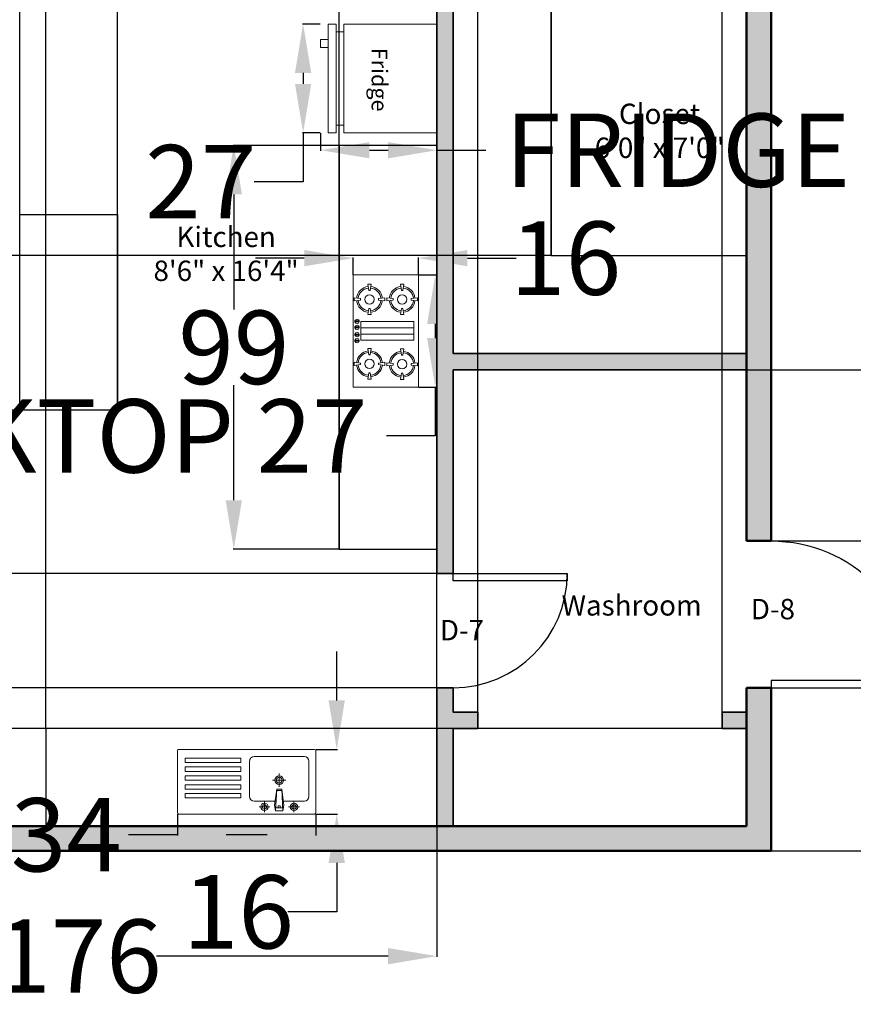
# Model space of a CAD drawing. Units: inches. Extents: x -478 to 256, y -93 to 343.
# Tile 3 of 5: x -106 to 98, y -93 to 149. Entities that reach past the tile are written whole.
import ezdxf

# ---------------------------------------------------------------- set-up
doc = ezdxf.new("R2010")
doc.units = ezdxf.units.IN
for name, color, linetype, lineweight in [('A-ANNO-DIMS', 2, 'Continuous', 18), ('A-ANNO-TEXT', 7, 'Continuous', 18), ('A-AREA-IDEN', 7, 'Continuous', 18), ('A-DOOR', 3, 'Continuous', 25), ('A-EQPM', 6, 'Continuous', 18), ('A-FLOR-CASE', 6, 'Continuous', 25), ('A-FLOR-FIXT', 9, 'Continuous', 18), ('A-WALL-PATT', 8, 'Continuous', 13), ('Inner Wall', 5, 'Continuous', 35), ('Outer Wall', 1, 'Continuous', 50)]:
    doc.layers.add(name, color=color, linetype=linetype, lineweight=lineweight)
doc.styles.get("Standard").update_dxf_attribs({"font": 'arial.ttf'})
doc.dimstyles.get("Standard").update_dxf_attribs({"dimtxt": 18, "dimasz": 12, "dimexe": 0.18, "dimexo": 0.0625, "dimgap": 0.09, "dimtad": 0, "dimtih": 1, "dimtoh": 1, "dimdec": 0, "dimzin": 0, "dimdsep": 46, "dimlunit": 3, "dimtxsty": 'Standard', "dimcen": 0.09, "dimadec": 0, "dimazin": 0, "dimtfac": 1, "dimtdec": 0, "dimtofl": 0, "dimtmove": 0, "dimatfit": 3, "dimfxl": 1, "dimtolj": 1, "dimtzin": 0, "dimarcsym": 0})

# ---------------------------------------------------------------- blocks, each defined once
blk = doc.blocks.new('REFRI-00')
for points in [[(-0.35, 0.35), (-0.35, -0.25), (0.35, -0.25), (0.35, 0.35), (-0.35, 0.35)], [(-0.3, -0.3), (-0.3, -0.25)], [(0.3, -0.3), (0.3, -0.25)], [(-0.35, -0.3), (-0.35, -0.35), (0.35, -0.35), (0.35, -0.3), (-0.35, -0.3)], [(-0.25, -0.35), (-0.25, -0.4), (-0.2, -0.4), (-0.2, -0.35)]]:
    blk.add_lwpolyline(points)
blk = doc.blocks.new('A$C57CF26DA')
for p, q in [((0, 0), (0, 420)), ((720, 420), (0, 420)), ((166.9, 413), (146.9, 413)), ((146.9, 413), (151.9, 373)), ((161.9, 373), (166.9, 413)), ((300, 390.9), (300, 49.1)), ((300, 390.9), (420, 390.9)), ((340, 390.9), (340, 49.1)), ((380, 390.9), (380, 49.1)), ((420, 390.9), (420, 49.1)), ((583.6, 413), (563.6, 413)), ((563.6, 413), (568.6, 373)), ((578.6, 373), (583.6, 413)), ((720, 0), (720, 420)), ((98.9, 320), (58.9, 325)), ((58.9, 325), (58.9, 305)), ((98.9, 310), (98.9, 320)), ((151.9, 373), (161.9, 373)), ((254.8, 325), (214.8, 320)), ((214.8, 320), (214.8, 310)), ((254.8, 305), (254.8, 325)), ((515.6, 320), (475.6, 325)), ((475.6, 325), (475.6, 305)), ((515.6, 310), (515.6, 320)), ((568.6, 373), (578.6, 373)), ((671.6, 325), (631.6, 320)), ((631.6, 320), (631.6, 310)), ((671.6, 305), (671.6, 325)), ((58.9, 305), (98.9, 310)), ((151.9, 257), (146.9, 217)), ((161.9, 257), (151.9, 257)), ((166.9, 217), (161.9, 257)), ((214.8, 310), (254.8, 305)), ((475.6, 305), (515.6, 310)), ((568.6, 257), (563.6, 217)), ((578.6, 257), (568.6, 257)), ((583.6, 217), (578.6, 257)), ((631.6, 310), (671.6, 305)), ((146.9, 217), (166.9, 217)), ((166.9, 203), (146.9, 203)), ((146.9, 203), (151.9, 163)), ((161.9, 163), (166.9, 203)), ((581.1, 203), (561.1, 203)), ((561.1, 203), (566.1, 163)), ((563.6, 217), (583.6, 217)), ((576.1, 163), (581.1, 203)), ((151.9, 163), (161.9, 163)), ((566.1, 163), (576.1, 163)), ((98.9, 110), (58.9, 115)), ((58.9, 115), (58.9, 95)), ((58.9, 95), (98.9, 100)), ((98.9, 100), (98.9, 110)), ((254.8, 115), (214.8, 110)), ((214.8, 110), (214.8, 100)), ((214.8, 100), (254.8, 95)), ((254.8, 95), (254.8, 115)), ((513.1, 110), (473.1, 115)), ((473.1, 115), (473.1, 95)), ((473.1, 95), (513.1, 100)), ((513.1, 100), (513.1, 110)), ((669, 115), (629, 110)), ((629, 110), (629, 100)), ((629, 100), (669, 95)), ((669, 95), (669, 115)), ((151.9, 47), (146.9, 7)), ((146.9, 7), (166.9, 7)), ((161.9, 47), (151.9, 47)), ((166.9, 7), (161.9, 47)), ((301.5, 38.7), (294.7, 38.7)), ((294.7, 38.7), (294.7, 11.3)), ((294.7, 11.3), (301.5, 11.3)), ((420, 49.1), (300, 49.1)), ((301.5, 11.3), (301.5, 38.7)), ((340.5, 38.7), (333.7, 38.7)), ((333.7, 38.7), (333.7, 11.3)), ((333.7, 11.3), (340.5, 11.3)), ((340.5, 11.3), (340.5, 38.7)), ((379.7, 11.3), (379.7, 38.7)), ((379.7, 38.7), (386.5, 38.7)), ((386.5, 11.3), (379.7, 11.3)), ((386.5, 38.7), (386.5, 11.3)), ((418.7, 11.3), (418.7, 38.7)), ((418.7, 38.7), (425.5, 38.7)), ((425.5, 11.3), (418.7, 11.3)), ((425.5, 38.7), (425.5, 11.3)), ((566.1, 47), (561.1, 7)), ((561.1, 7), (581.1, 7)), ((576.1, 47), (566.1, 47)), ((581.1, 7), (576.1, 47)), ((720, 0), (0, 0))]:
    blk.add_line(p, q)
for centre in [(156.9, 315), (573.6, 315), (156.9, 105), (571.1, 105)]:
    blk.add_circle(centre, 30)
for centre, radius, start, end in [((156.9, 315), 83, 95.58493, 174.41507), ((156.9, 315), 73, 95.37384, 174.62616), ((156.9, 315), 73, 5.37384, 84.62616), ((156.9, 315), 83, 5.58493, 84.41507), ((573.6, 315), 83, 95.58493, 174.41507), ((573.6, 315), 73, 95.37384, 174.62616), ((573.6, 315), 73, 5.37384, 84.62616), ((573.6, 315), 83, 5.58493, 84.41507), ((156.9, 315), 83, 185.58493, 264.41507), ((156.9, 315), 73, 185.37384, 264.62616), ((156.9, 315), 73, 275.37384, 354.62616), ((156.9, 315), 83, 275.58493, 354.41507), ((573.6, 315), 83, 185.58493, 264.41507), ((573.6, 315), 73, 185.37384, 264.62616), ((573.6, 315), 73, 275.37384, 354.62616), ((573.6, 315), 83, 275.58493, 354.41507), ((156.9, 105), 83, 95.58493, 174.41507), ((156.9, 105), 73, 95.37384, 174.62616), ((156.9, 105), 73, 5.37384, 84.62616), ((156.9, 105), 83, 5.58493, 84.41507), ((571.1, 105), 83, 95.58493, 174.41507), ((571.1, 105), 73, 95.37384, 174.62616), ((571.1, 105), 73, 5.37384, 84.62616), ((571.1, 105), 83, 5.58493, 84.41507), ((156.9, 105), 83, 185.58493, 264.41507), ((156.9, 105), 73, 185.37384, 264.62616), ((156.9, 105), 73, 275.37384, 354.62616), ((156.9, 105), 83, 275.58493, 354.41507), ((571.1, 105), 83, 185.58493, 264.41507), ((571.1, 105), 73, 185.37384, 264.62616), ((571.1, 105), 73, 275.37384, 354.62616), ((571.1, 105), 83, 275.58493, 354.41507), ((298.1, 25), 13.7, 104.47751, 255.52249), ((298.1, 25), 13.7, 284.47751, 75.52249), ((337.1, 25), 13.7, 104.47751, 255.52249), ((337.1, 25), 13.7, 284.47751, 75.52249), ((383.1, 25), 13.7, 104.47751, 255.52249), ((383.1, 25), 13.7, 284.47751, 75.52249), ((422.1, 25), 13.7, 104.47751, 255.52249), ((422.1, 25), 13.7, 284.47751, 75.52249)]:
    blk.add_arc(centre, radius, start, end)
blk = doc.blocks.new('A$C7C492201')
for p, q in [((0, 10), (0, 426.6)), ((10, 436.6), (927.3, 436.6)), ((148.5, 425.2), (148.5, 352.2)), ((223.5, 415), (217, 376.2)), ((223.5, 415), (231.8, 268.5)), ((223.5, 415), (248.5, 415)), ((273.5, 415), (248.5, 415)), ((273.5, 415), (265.2, 268.5)), ((273.5, 415), (279.9, 376.2)), ((348.5, 425.2), (348.5, 352.2)), ((937.3, 10), (937.3, 426.6)), ((220.8, 348.8), (78.5, 348.8)), ((111.9, 388.7), (185, 388.7)), ((217, 376.2), (231.8, 268.5)), ((224.6, 395.4), (248.5, 395.4)), ((272.3, 395.4), (248.5, 395.4)), ((279.9, 376.2), (265.2, 268.5)), ((418.5, 348.8), (276.2, 348.8)), ((311.9, 388.7), (385, 388.7)), ((48.5, 318.8), (48.5, 78.8)), ((231.3, 278.6), (248.5, 278.6)), ((231.8, 268.5), (248.5, 268.5)), ((265.6, 278.6), (248.5, 278.6)), ((265.2, 268.5), (248.5, 268.5)), ((448.5, 318.8), (448.5, 78.8)), ((509.1, 328.4), (509.1, 298.4)), ((509.1, 328.4), (885, 328.4)), ((509.1, 298.4), (885, 298.4)), ((509.1, 268.4), (509.1, 238.4)), ((509.1, 268.4), (885, 268.4)), ((885, 328.4), (885, 298.4)), ((885, 268.4), (885, 238.4)), ((203.4, 207.7), (293.5, 207.7)), ((248.5, 252.8), (248.5, 162.6)), ((509.1, 238.4), (885, 238.4)), ((509.1, 208.4), (885, 208.4)), ((509.1, 208.4), (509.1, 178.4)), ((885, 208.4), (885, 178.4)), ((509.1, 178.4), (885, 178.4)), ((509.1, 148.4), (509.1, 118.4)), ((509.1, 148.4), (885, 148.4)), ((885, 148.4), (885, 118.4)), ((509.1, 118.4), (885, 118.4)), ((509.1, 88.4), (509.1, 58.4)), ((509.1, 88.4), (885, 88.4)), ((885, 88.4), (885, 58.4)), ((927.3, 0), (10, 0)), ((418.5, 48.8), (78.5, 48.8)), ((509.1, 58.4), (885, 58.4))]:
    blk.add_line(p, q)
for centre, radius in [((148.5, 388.7), 25), ((148.5, 388.7), 15), ((348.5, 388.7), 25), ((348.5, 388.7), 15), ((248.5, 207.7), 30), ((248.5, 207.7), 20)]:
    blk.add_circle(centre, radius)
for centre, radius, start, end in [((10, 426.6), 10, 90, 180), ((927.3, 426.6), 10, 0, 90), ((78.5, 318.8), 30, 90, 180), ((247.3, 388), 7.19, 80.52523, 279.47477), ((249.6, 388), 7.19, 260.52523, 99.47477), ((418.5, 318.8), 30, 0, 90), ((78.5, 78.8), 30, 180, 270), ((418.5, 78.8), 30, 270, 0), ((10, 10), 10, 180, 270), ((927.3, 10), 10, 270, 0)]:
    blk.add_arc(centre, radius, start, end)
blk = doc.blocks.new('*U4')
for p, q in [((0, 0), (0, -4)), ((28, 0), (28, -4))]:
    blk.add_line(p, q)
blk.add_lwpolyline([(0, 0), (0, 28), (1.75, 28), (1.75, 0)], close=True)
blk.add_arc((0, 0), 28, 0, 90)
blk = doc.blocks.new('*U14')
for p, q in [((0, 0), (0, -6)), ((36, 0), (36, -6))]:
    blk.add_line(p, q)
blk.add_lwpolyline([(0, 0), (0, 36), (1.75, 36), (1.75, 0)], close=True)
blk.add_arc((0, 0), 36, 0, 90)
blk = doc.blocks.new('*D17')
at = {"layer": 'A-ANNO-DIMS', "color": 0, "lineweight": -2, "transparency": 16777216}
for p, q in [((-32.43, 120.92), (-32.43, 116.52)), ((-3.86, 120.92), (-3.86, 116.52)), ((-20.43, 116.7), (-15.86, 116.7)), ((-3.86, 116.7), (8.14, 116.7))]:
    blk.add_line(p, q, dxfattribs=at)
at = {"layer": 'A-ANNO-DIMS', "color": 0, "transparency": 16777216}
for points in [[(-20.43, 118.7), (-20.43, 114.7), (-32.43, 116.7)], [(-15.86, 118.7), (-15.86, 114.7), (-3.86, 116.7)]]:
    blk.add_solid(points, dxfattribs=at)
at = {"layer": 'Defpoints', "color": 0, "transparency": 16777216}
for p in [(-32.43, 120.98), (-3.86, 120.98), (-3.86, 116.7)]:
    blk.add_point(p, dxfattribs=at)
at = {"layer": 'A-ANNO-DIMS', "color": 0, "transparency": 16777216, "insert": (71.63, 116.7), "char_height": 18, "attachment_point": 5}
blk.add_mtext('\\A1;FRIDGE 29', dxfattribs=at)
blk = doc.blocks.new('*D18')
at = {"layer": 'A-ANNO-DIMS', "color": 0, "lineweight": -2, "transparency": 16777216}
for p, q in [((-32.49, 147.65), (-36.89, 147.65)), ((-36.71, 135.65), (-36.71, 132.98)), ((-32.49, 120.98), (-36.89, 120.98)), ((-36.71, 120.98), (-36.71, 108.98)), ((-36.71, 108.98), (-48.71, 108.98))]:
    blk.add_line(p, q, dxfattribs=at)
at = {"layer": 'A-ANNO-DIMS', "color": 0, "transparency": 16777216}
for points in [[(-38.71, 135.65), (-34.71, 135.65), (-36.71, 147.65)], [(-38.71, 132.98), (-34.71, 132.98), (-36.71, 120.98)]]:
    blk.add_solid(points, dxfattribs=at)
at = {"layer": 'Defpoints', "color": 0, "transparency": 16777216}
for p in [(-32.43, 147.65), (-36.71, 120.98), (-32.43, 120.98)]:
    blk.add_point(p, dxfattribs=at)
at = {"layer": 'A-ANNO-DIMS', "color": 0, "transparency": 16777216, "insert": (-61.85, 108.98), "char_height": 18, "attachment_point": 5}
blk.add_mtext('\\A1;27', dxfattribs=at)
blk = doc.blocks.new('*D19')
at = {"layer": 'A-ANNO-DIMS', "color": 0, "lineweight": -2, "transparency": 16777216}
for p, q in [((-8.33, 86.09), (-4.09, 86.09)), ((-4.27, 74.09), (-4.27, 70.61)), ((-8.33, 58.61), (-4.09, 58.61)), ((-4.27, 58.61), (-4.27, 46.61)), ((-4.27, 46.61), (-16.27, 46.61))]:
    blk.add_line(p, q, dxfattribs=at)
at = {"layer": 'A-ANNO-DIMS', "color": 0, "transparency": 16777216}
for points in [[(-6.27, 74.09), (-2.27, 74.09), (-4.27, 86.09)], [(-6.27, 70.61), (-2.27, 70.61), (-4.27, 58.61)]]:
    blk.add_solid(points, dxfattribs=at)
at = {"layer": 'Defpoints', "color": 0, "transparency": 16777216}
for p in [(-8.39, 86.09), (-8.39, 58.61), (-4.27, 58.61)]:
    blk.add_point(p, dxfattribs=at)
at = {"layer": 'A-ANNO-DIMS', "color": 0, "transparency": 16777216, "insert": (-95.51, 46.61), "char_height": 18, "attachment_point": 5}
blk.add_mtext('\\A1;COOKTOP 27', dxfattribs=at)
blk = doc.blocks.new('*D20')
at = {"layer": 'A-ANNO-DIMS', "color": 0, "lineweight": -2, "transparency": 16777216}
for p, q in [((-36.42, 90.22), (-48.42, 90.22)), ((-24.42, 86.16), (-24.42, 90.4)), ((-8.39, 86.16), (-8.39, 90.4)), ((3.61, 90.22), (15.61, 90.22))]:
    blk.add_line(p, q, dxfattribs=at)
at = {"layer": 'A-ANNO-DIMS', "color": 0, "transparency": 16777216}
for points in [[(-36.42, 92.22), (-36.42, 88.22), (-24.42, 90.22)], [(3.61, 92.22), (3.61, 88.22), (-8.39, 90.22)]]:
    blk.add_solid(points, dxfattribs=at)
at = {"layer": 'Defpoints', "color": 0, "transparency": 16777216}
for p in [(-8.39, 90.22), (-24.42, 86.09), (-8.39, 86.09)]:
    blk.add_point(p, dxfattribs=at)
at = {"layer": 'A-ANNO-DIMS', "color": 0, "transparency": 16777216, "insert": (27.74, 90.22), "char_height": 18, "attachment_point": 5}
blk.add_mtext('\\A1;16', dxfattribs=at)
blk = doc.blocks.new('*D21')
at = {"layer": 'A-ANNO-DIMS', "color": 0, "lineweight": -2, "transparency": 16777216}
for p, q in [((-67.57, -46.21), (-67.57, -51.43)), ((-33.56, -46.21), (-33.56, -51.43)), ((-67.57, -51.25), (-79.57, -51.25)), ((-45.56, -51.25), (-55.57, -51.25))]:
    blk.add_line(p, q, dxfattribs=at)
at = {"layer": 'A-ANNO-DIMS', "color": 0, "transparency": 16777216}
for points in [[(-55.57, -49.25), (-55.57, -53.25), (-67.57, -51.25)], [(-45.56, -49.25), (-45.56, -53.25), (-33.56, -51.25)]]:
    blk.add_solid(points, dxfattribs=at)
at = {"layer": 'Defpoints', "color": 0, "transparency": 16777216}
for p in [(-67.57, -46.15), (-33.56, -46.15), (-67.57, -51.25)]:
    blk.add_point(p, dxfattribs=at)
at = {"layer": 'A-ANNO-DIMS', "color": 0, "transparency": 16777216, "insert": (-125.31, -51.25), "char_height": 18, "attachment_point": 5}
blk.add_mtext('\\A1;SINK 34', dxfattribs=at)
blk = doc.blocks.new('*D22')
at = {"layer": 'A-ANNO-DIMS', "color": 0, "lineweight": -2, "transparency": 16777216}
for p, q in [((-28.46, -18.3), (-28.46, -6.3)), ((-33.5, -30.3), (-28.28, -30.3)), ((-33.5, -46.15), (-28.28, -46.15)), ((-28.46, -58.15), (-28.46, -70.15)), ((-28.46, -70.15), (-40.46, -70.15))]:
    blk.add_line(p, q, dxfattribs=at)
at = {"layer": 'A-ANNO-DIMS', "color": 0, "transparency": 16777216}
for points in [[(-30.46, -18.3), (-26.46, -18.3), (-28.46, -30.3)], [(-30.46, -58.15), (-26.46, -58.15), (-28.46, -46.15)]]:
    blk.add_solid(points, dxfattribs=at)
at = {"layer": 'Defpoints', "color": 0, "transparency": 16777216}
for p in [(-33.56, -30.3), (-33.56, -46.15), (-28.46, -46.15)]:
    blk.add_point(p, dxfattribs=at)
at = {"layer": 'A-ANNO-DIMS', "color": 0, "transparency": 16777216, "insert": (-52.59, -70.15), "char_height": 18, "attachment_point": 5}
blk.add_mtext('\\A1;16', dxfattribs=at)
blk = doc.blocks.new('*D27')
at = {"layer": 'A-ANNO-DIMS', "color": 0, "lineweight": -2, "transparency": 16777216}
for p, q in [((-56.12, 205.87), (-56.12, 189.02)), ((55.39, 205.87), (55.39, 189.02)), ((-44.12, 189.2), (43.39, 189.2)), ((55.39, 189.2), (67.39, 189.2))]:
    blk.add_line(p, q, dxfattribs=at)
at = {"layer": 'A-ANNO-DIMS', "color": 0, "transparency": 16777216}
for points in [[(-44.12, 191.2), (-44.12, 187.2), (-56.12, 189.2)], [(43.39, 191.2), (43.39, 187.2), (55.39, 189.2)]]:
    blk.add_solid(points, dxfattribs=at)
at = {"layer": 'Defpoints', "color": 0, "transparency": 16777216}
for p in [(-56.12, 205.93), (55.39, 205.93), (55.39, 189.2)]:
    blk.add_point(p, dxfattribs=at)
at = {"layer": 'A-ANNO-DIMS', "color": 0, "transparency": 16777216, "insert": (165.82, 189.2), "char_height": 18, "attachment_point": 5}
blk.add_mtext('\\A1;BED GROUP 112', dxfattribs=at)
blk = doc.blocks.new('*D35')
at = {"layer": 'A-ANNO-DIMS', "color": 0, "lineweight": -2, "transparency": 16777216}
for p, q in [((-3.86, -49.22), (-3.86, -81.2)), ((-179.86, -55.22), (-179.86, -81.2)), ((-167.86, -81.02), (-110.98, -81.02)), ((-15.86, -81.02), (-72.73, -81.02))]:
    blk.add_line(p, q, dxfattribs=at)
at = {"layer": 'A-ANNO-DIMS', "color": 0, "transparency": 16777216}
for points in [[(-167.86, -79.02), (-167.86, -83.02), (-179.86, -81.02)], [(-15.86, -79.02), (-15.86, -83.02), (-3.86, -81.02)]]:
    blk.add_solid(points, dxfattribs=at)
at = {"layer": 'Defpoints', "color": 0, "transparency": 16777216}
for p in [(-3.86, -49.16), (-179.86, -55.16), (-3.86, -81.02)]:
    blk.add_point(p, dxfattribs=at)
at = {"layer": 'A-ANNO-DIMS', "color": 0, "transparency": 16777216, "insert": (-91.86, -81.02), "char_height": 18, "attachment_point": 5}
blk.add_mtext('\\A1;176', dxfattribs=at)
blk = doc.blocks.new('*D39')
at = {"layer": 'A-ANNO-DIMS', "color": 0, "lineweight": -2, "transparency": 16777216}
for p, q in [((140.01, -15.16), (140.01, -3.16)), ((140.01, -3.16), (152.01, -3.16)), ((78.21, -15.16), (140.19, -15.16)), ((140.01, -43.16), (140.01, -27.16)), ((78.21, -55.16), (140.19, -55.16))]:
    blk.add_line(p, q, dxfattribs=at)
at = {"layer": 'A-ANNO-DIMS', "color": 0, "transparency": 16777216}
for points in [[(138.01, -27.16), (142.01, -27.16), (140.01, -15.16)], [(138.01, -43.16), (142.01, -43.16), (140.01, -55.16)]]:
    blk.add_solid(points, dxfattribs=at)
at = {"layer": 'Defpoints', "color": 0, "transparency": 16777216}
for p in [(78.14, -15.16), (140.01, -15.16), (78.14, -55.16)]:
    blk.add_point(p, dxfattribs=at)
at = {"layer": 'A-ANNO-DIMS', "color": 0, "transparency": 16777216, "insert": (165.32, -3.16), "char_height": 18, "attachment_point": 5}
blk.add_mtext('\\A1;40', dxfattribs=at)
blk = doc.blocks.new('*D40')
at = {"layer": 'A-ANNO-DIMS', "color": 0, "lineweight": -2, "transparency": 16777216}
for p, q in [((140.01, 20.84), (140.01, 32.84)), ((140.01, 32.84), (152.01, 32.84)), ((78.21, 20.84), (140.19, 20.84)), ((140.01, -3.16), (140.01, 8.84)), ((78.21, -15.16), (140.19, -15.16))]:
    blk.add_line(p, q, dxfattribs=at)
at = {"layer": 'A-ANNO-DIMS', "color": 0, "transparency": 16777216}
for points in [[(138.01, 8.84), (142.01, 8.84), (140.01, 20.84)], [(138.01, -3.16), (142.01, -3.16), (140.01, -15.16)]]:
    blk.add_solid(points, dxfattribs=at)
at = {"layer": 'Defpoints', "color": 0, "transparency": 16777216}
for p in [(78.14, 20.84), (140.01, 20.84), (78.14, -15.16)]:
    blk.add_point(p, dxfattribs=at)
at = {"layer": 'A-ANNO-DIMS', "color": 0, "transparency": 16777216, "insert": (164.98, 32.84), "char_height": 18, "attachment_point": 5}
blk.add_mtext('\\A1;36', dxfattribs=at)
blk = doc.blocks.new('*D41')
at = {"layer": 'A-ANNO-DIMS', "color": 0, "lineweight": -2, "transparency": 16777216}
for p, q in [((140.01, 62.84), (140.01, 74.84)), ((140.01, 74.84), (152.01, 74.84)), ((72.21, 62.84), (140.19, 62.84)), ((140.01, 32.84), (140.01, 50.84)), ((78.21, 20.84), (140.19, 20.84))]:
    blk.add_line(p, q, dxfattribs=at)
at = {"layer": 'A-ANNO-DIMS', "color": 0, "transparency": 16777216}
for points in [[(138.01, 50.84), (142.01, 50.84), (140.01, 62.84)], [(138.01, 32.84), (142.01, 32.84), (140.01, 20.84)]]:
    blk.add_solid(points, dxfattribs=at)
at = {"layer": 'Defpoints', "color": 0, "transparency": 16777216}
for p in [(72.14, 62.84), (140.01, 62.84), (78.14, 20.84)]:
    blk.add_point(p, dxfattribs=at)
at = {"layer": 'A-ANNO-DIMS', "color": 0, "transparency": 16777216, "insert": (165.26, 74.84), "char_height": 18, "attachment_point": 5}
blk.add_mtext('\\A1;42', dxfattribs=at)
blk = doc.blocks.new('*D52')
at = {"layer": 'A-ANNO-DIMS', "color": 0, "lineweight": -2, "transparency": 16777216}
for p, q in [((-427.72, 12.84), (-427.72, 24.84)), ((-427.72, 24.84), (-415.72, 24.84)), ((0.08, 12.84), (-427.9, 12.84)), ((-427.72, -3.16), (-427.72, 0.84)), ((0.08, -15.16), (-427.9, -15.16))]:
    blk.add_line(p, q, dxfattribs=at)
at = {"layer": 'A-ANNO-DIMS', "color": 0, "transparency": 16777216}
for points in [[(-429.72, 0.84), (-425.72, 0.84), (-427.72, 12.84)], [(-429.72, -3.16), (-425.72, -3.16), (-427.72, -15.16)]]:
    blk.add_solid(points, dxfattribs=at)
at = {"layer": 'Defpoints', "color": 0, "transparency": 16777216}
for p in [(-427.72, 12.84), (0.14, 12.84), (0.14, -15.16)]:
    blk.add_point(p, dxfattribs=at)
at = {"layer": 'A-ANNO-DIMS', "color": 0, "transparency": 16777216, "insert": (-402.57, 24.84), "char_height": 18, "attachment_point": 5}
blk.add_mtext('\\A1;28', dxfattribs=at)
blk = doc.blocks.new('*D53')
at = {"layer": 'A-ANNO-DIMS', "color": 0, "lineweight": -2, "transparency": 16777216}
for p, q in [((-118.28, 330.71), (-130.28, 330.71)), ((-106.28, 101.01), (-106.28, 330.89)), ((-82.28, 101.01), (-82.28, 330.89)), ((-70.28, 330.71), (-58.28, 330.71))]:
    blk.add_line(p, q, dxfattribs=at)
at = {"layer": 'A-ANNO-DIMS', "color": 0, "transparency": 16777216}
for points in [[(-118.28, 332.71), (-118.28, 328.71), (-106.28, 330.71)], [(-70.28, 332.71), (-70.28, 328.71), (-82.28, 330.71)]]:
    blk.add_solid(points, dxfattribs=at)
at = {"layer": 'Defpoints', "color": 0, "transparency": 16777216}
for p in [(-82.28, 330.71), (-106.28, 100.95), (-82.28, 100.95)]:
    blk.add_point(p, dxfattribs=at)
at = {"layer": 'A-ANNO-DIMS', "color": 0, "transparency": 16777216, "insert": (-45.18, 330.71), "char_height": 18, "attachment_point": 5}
blk.add_mtext('\\A1;24', dxfattribs=at)
blk = doc.blocks.new('*D57')
at = {"layer": 'A-ANNO-DIMS', "color": 0, "lineweight": -2, "transparency": 16777216}
for p, q in [((-99.86, -25.1), (-99.86, 330.89)), ((-87.86, 330.71), (-64.83, 330.71)), ((-15.86, 330.71), (-38.88, 330.71)), ((-3.86, -25.1), (-3.86, 330.89))]:
    blk.add_line(p, q, dxfattribs=at)
at = {"layer": 'A-ANNO-DIMS', "color": 0, "transparency": 16777216}
for points in [[(-87.86, 332.71), (-87.86, 328.71), (-99.86, 330.71)], [(-15.86, 332.71), (-15.86, 328.71), (-3.86, 330.71)]]:
    blk.add_solid(points, dxfattribs=at)
at = {"layer": 'Defpoints', "color": 0, "transparency": 16777216}
for p in [(-3.86, 330.71), (-99.86, -25.16), (-3.86, -25.16)]:
    blk.add_point(p, dxfattribs=at)
at = {"layer": 'A-ANNO-DIMS', "color": 0, "transparency": 16777216, "insert": (-51.86, 330.71), "char_height": 18, "attachment_point": 5}
blk.add_mtext('\\A1;96', dxfattribs=at)
blk = doc.blocks.new('*D58')
at = {"layer": 'A-ANNO-DIMS', "color": 0, "lineweight": -2, "transparency": 16777216}
for p, q in [((-427.720811, -13.158903), (-427.720811, -1.158903)), ((-99.918311, -25.158903), (-427.900811, -25.158903)), ((-99.918311, -49.158903), (-427.900811, -49.158903)), ((-427.720811, -61.158903), (-427.720811, -73.158903))]:
    blk.add_line(p, q, dxfattribs=at)
at = {"layer": 'A-ANNO-DIMS', "color": 0, "transparency": 16777216}
for points in [[(-429.720811, -13.158903), (-425.720811, -13.158903), (-427.720811, -25.158903)], [(-429.720811, -61.158903), (-425.720811, -61.158903), (-427.720811, -49.158903)]]:
    blk.add_solid(points, dxfattribs=at)
at = {"layer": 'Defpoints', "color": 0, "transparency": 16777216}
for p in [(-427.720811, -25.158903), (-99.855811, -25.158903), (-99.855811, -49.158903)]:
    blk.add_point(p, dxfattribs=at)
at = {"layer": 'A-ANNO-DIMS', "color": 0, "transparency": 16777216, "insert": (-427.720811, -37.158903), "char_height": 18, "attachment_point": 5}
blk.add_mtext('\\A1;24', dxfattribs=at)
blk = doc.blocks.new('*D59')
at = {"layer": 'A-ANNO-DIMS', "color": 0, "lineweight": -2, "transparency": 16777216}
for p, q in [((-27.92, 117.84), (-53.9, 117.84)), ((-53.72, 105.84), (-53.72, 77.62)), ((-53.72, 30.84), (-53.72, 59.06)), ((-27.92, 18.84), (-53.9, 18.84))]:
    blk.add_line(p, q, dxfattribs=at)
at = {"layer": 'A-ANNO-DIMS', "color": 0, "transparency": 16777216}
for points in [[(-55.72, 105.84), (-51.72, 105.84), (-53.72, 117.84)], [(-55.72, 30.84), (-51.72, 30.84), (-53.72, 18.84)]]:
    blk.add_solid(points, dxfattribs=at)
at = {"layer": 'Defpoints', "color": 0, "transparency": 16777216}
for p in [(-53.72, 117.84), (-27.86, 117.84), (-27.86, 18.84)]:
    blk.add_point(p, dxfattribs=at)
at = {"layer": 'A-ANNO-DIMS', "color": 0, "transparency": 16777216, "insert": (-53.72, 68.34), "char_height": 18, "attachment_point": 5}
blk.add_mtext('\\A1;99', dxfattribs=at)
blk = doc.blocks.new('*D60')
at = {"layer": 'A-ANNO-DIMS', "color": 0, "lineweight": -2, "transparency": 16777216}
for p, q in [((-39.86, 330.71), (-51.86, 330.71)), ((-27.86, 18.9), (-27.86, 330.89)), ((-3.86, 18.9), (-3.86, 330.89)), ((8.14, 330.71), (20.14, 330.71))]:
    blk.add_line(p, q, dxfattribs=at)
at = {"layer": 'A-ANNO-DIMS', "color": 0, "transparency": 16777216}
for points in [[(-39.86, 332.71), (-39.86, 328.71), (-27.86, 330.71)], [(8.14, 332.71), (8.14, 328.71), (-3.86, 330.71)]]:
    blk.add_solid(points, dxfattribs=at)
at = {"layer": 'Defpoints', "color": 0, "transparency": 16777216}
for p in [(-3.86, 330.71), (-27.86, 18.84), (-3.86, 18.84)]:
    blk.add_point(p, dxfattribs=at)
at = {"layer": 'A-ANNO-DIMS', "color": 0, "transparency": 16777216, "insert": (33.24, 330.71), "char_height": 18, "attachment_point": 5}
blk.add_mtext('\\A1;24', dxfattribs=at)
blk = doc.blocks.new('*D61')
at = {"layer": 'A-ANNO-DIMS', "color": 0, "lineweight": -2, "transparency": 16777216}
for p, q in [((-106.35, 52.95), (-427.9, 52.95)), ((-427.72, 40.95), (-427.72, 23.18)), ((-427.72, -13.16), (-427.72, 4.61)), ((-99.92, -25.16), (-427.9, -25.16))]:
    blk.add_line(p, q, dxfattribs=at)
at = {"layer": 'A-ANNO-DIMS', "color": 0, "transparency": 16777216}
for points in [[(-429.72, 40.95), (-425.72, 40.95), (-427.72, 52.95)], [(-429.72, -13.16), (-425.72, -13.16), (-427.72, -25.16)]]:
    blk.add_solid(points, dxfattribs=at)
at = {"layer": 'Defpoints', "color": 0, "transparency": 16777216}
for p in [(-427.72, 52.95), (-106.28, 52.95), (-99.86, -25.16)]:
    blk.add_point(p, dxfattribs=at)
at = {"layer": 'A-ANNO-DIMS', "color": 0, "transparency": 16777216, "insert": (-427.72, 13.9), "char_height": 18, "attachment_point": 5}
blk.add_mtext('\\A1;78.11', dxfattribs=at)
blk = doc.blocks.new('*D62')
at = {"layer": 'A-ANNO-DIMS', "color": 0, "lineweight": -2, "transparency": 16777216}
for p, q in [((-82.28, 53.01), (-82.28, 330.89)), ((-70.28, 330.71), (-39.86, 330.71)), ((-27.86, 18.9), (-27.86, 330.89)), ((-27.86, 330.71), (-15.86, 330.71))]:
    blk.add_line(p, q, dxfattribs=at)
at = {"layer": 'A-ANNO-DIMS', "color": 0, "transparency": 16777216}
for points in [[(-70.28, 332.71), (-70.28, 328.71), (-82.28, 330.71)], [(-39.86, 332.71), (-39.86, 328.71), (-27.86, 330.71)]]:
    blk.add_solid(points, dxfattribs=at)
at = {"layer": 'Defpoints', "color": 0, "transparency": 16777216}
for p in [(-27.86, 330.71), (-82.28, 52.95), (-27.86, 18.84)]:
    blk.add_point(p, dxfattribs=at)
at = {"layer": 'A-ANNO-DIMS', "color": 0, "transparency": 16777216, "insert": (14.6, 330.71), "char_height": 18, "attachment_point": 5}
blk.add_mtext('\\A1;54.43', dxfattribs=at)
blk = doc.blocks.new('*D65')
at = {"layer": 'A-ANNO-DIMS', "color": 0, "lineweight": -2, "transparency": 16777216}
for p, q in [((12.144189, 330.706097), (0.144189, 330.706097)), ((24.144189, 90.903597), (24.144189, 330.886097)), ((72.144189, 90.903597), (72.144189, 330.886097)), ((84.144189, 330.706097), (96.144189, 330.706097))]:
    blk.add_line(p, q, dxfattribs=at)
at = {"layer": 'A-ANNO-DIMS', "color": 0, "transparency": 16777216}
for points in [[(12.144189, 332.706097), (12.144189, 328.706097), (24.144189, 330.706097)], [(84.144189, 332.706097), (84.144189, 328.706097), (72.144189, 330.706097)]]:
    blk.add_solid(points, dxfattribs=at)
at = {"layer": 'Defpoints', "color": 0, "transparency": 16777216}
for p in [(72.144189, 330.706097), (24.144189, 90.841097), (72.144189, 90.841097)]:
    blk.add_point(p, dxfattribs=at)
at = {"layer": 'A-ANNO-DIMS', "color": 0, "transparency": 16777216, "insert": (48.144189, 330.706097), "char_height": 18, "attachment_point": 5}
blk.add_mtext('\\A1;48', dxfattribs=at)
blk = doc.blocks.new('*D66')
at = {"layer": 'A-ANNO-DIMS', "color": 0, "lineweight": -2, "transparency": 16777216}
for p, q in [((24.08, 150.84), (-427.9, 150.84)), ((-427.72, 138.84), (-427.72, 130.12)), ((-427.72, 102.84), (-427.72, 111.56)), ((24.08, 90.84), (-427.9, 90.84))]:
    blk.add_line(p, q, dxfattribs=at)
at = {"layer": 'A-ANNO-DIMS', "color": 0, "transparency": 16777216}
for points in [[(-429.72, 138.84), (-425.72, 138.84), (-427.72, 150.84)], [(-429.72, 102.84), (-425.72, 102.84), (-427.72, 90.84)]]:
    blk.add_solid(points, dxfattribs=at)
at = {"layer": 'Defpoints', "color": 0, "transparency": 16777216}
for p in [(-427.72, 150.84), (24.14, 150.84), (24.14, 90.84)]:
    blk.add_point(p, dxfattribs=at)
at = {"layer": 'A-ANNO-DIMS', "color": 0, "transparency": 16777216, "insert": (-427.72, 120.84), "char_height": 18, "attachment_point": 5}
blk.add_mtext('\\A1;60', dxfattribs=at)
blk = doc.blocks.new('*D67')
at = {"layer": 'A-ANNO-DIMS', "color": 0, "lineweight": -2, "transparency": 16777216}
for p, q in [((6.14, -25.1), (6.14, 330.89)), ((18.14, 330.71), (23.14, 330.71)), ((54.14, 330.71), (49.14, 330.71)), ((66.14, -25.1), (66.14, 330.89))]:
    blk.add_line(p, q, dxfattribs=at)
at = {"layer": 'A-ANNO-DIMS', "color": 0, "transparency": 16777216}
for points in [[(18.14, 332.71), (18.14, 328.71), (6.14, 330.71)], [(54.14, 332.71), (54.14, 328.71), (66.14, 330.71)]]:
    blk.add_solid(points, dxfattribs=at)
at = {"layer": 'Defpoints', "color": 0, "transparency": 16777216}
for p in [(66.14, 330.71), (6.14, -25.16), (66.14, -25.16)]:
    blk.add_point(p, dxfattribs=at)
at = {"layer": 'A-ANNO-DIMS', "color": 0, "transparency": 16777216, "insert": (36.14, 330.71), "char_height": 18, "attachment_point": 5}
blk.add_mtext('\\A1;60', dxfattribs=at)
blk = doc.blocks.new('*D68')
at = {"layer": 'A-ANNO-DIMS', "color": 0, "lineweight": -2, "transparency": 16777216}
for p, q in [((-427.720811, -13.158903), (-427.720811, -1.158903)), ((72.081689, -25.158903), (-427.900811, -25.158903)), ((72.081689, -49.158903), (-427.900811, -49.158903)), ((-427.720811, -61.158903), (-427.720811, -73.158903))]:
    blk.add_line(p, q, dxfattribs=at)
at = {"layer": 'A-ANNO-DIMS', "color": 0, "transparency": 16777216}
for points in [[(-429.720811, -13.158903), (-425.720811, -13.158903), (-427.720811, -25.158903)], [(-429.720811, -61.158903), (-425.720811, -61.158903), (-427.720811, -49.158903)]]:
    blk.add_solid(points, dxfattribs=at)
at = {"layer": 'Defpoints', "color": 0, "transparency": 16777216}
for p in [(-427.720811, -25.158903), (72.144189, -25.158903), (72.144189, -49.158903)]:
    blk.add_point(p, dxfattribs=at)
at = {"layer": 'A-ANNO-DIMS', "color": 0, "transparency": 16777216, "insert": (-427.720811, -37.158903), "char_height": 18, "attachment_point": 5}
blk.add_mtext('\\A1;24', dxfattribs=at)

msp = doc.modelspace()

# ---------------------------------------------------------------- hatches: boundary and pattern name
at = {"layer": 'A-WALL-PATT'}
h = msp.add_hatch(color=256, dxfattribs=at)
h.dxf.hatch_style = 1
h.paths.add_polyline_path([(-395.856, 298.841), (72.144, 298.841), (72.144, 20.841), (78.144, 20.841), (78.144, 304.841), (-401.856, 304.841), (-401.856, -55.159), (-215.856, -55.159), (-215.856, -49.159), (-395.856, -49.159)])
h.paths.add_polyline_path([(78.144, -15.159), (72.144, -15.159), (72.144, -49.159), (-179.856, -49.159), (-179.856, -55.159), (78.144, -55.159)], flags=17)
h = msp.add_hatch(color=256, dxfattribs=at)
h.dxf.hatch_style = 1
h.paths.add_polyline_path([(-329.856, 154.841), (-395.856, 154.841), (-395.856, 150.841), (-329.856, 150.841)])
h.paths.add_polyline_path([(-177.856, 154.841), (-243.856, 154.841), (-243.856, 160.841), (-247.856, 160.841), (-247.856, 154.841), (-283.856, 154.841), (-283.856, 224.841), (-247.856, 224.841), (-247.856, 218.841), (-243.856, 218.841), (-243.856, 298.841), (-247.856, 298.841), (-247.856, 228.841), (-283.856, 228.841), (-283.856, 234.841), (-287.856, 234.841), (-287.856, 154.841), (-293.856, 154.841), (-293.856, 150.841), (-177.856, 150.841)])
h.paths.add_polyline_path([(-283.856, 298.841), (-287.856, 298.841), (-287.856, 292.841), (-283.856, 292.841)], flags=17)
h.paths.add_polyline_path([(-131.856, 298.841), (-135.856, 298.841), (-135.856, 154.841), (-141.856, 154.841), (-141.856, 150.841), (-117.856, 150.841), (-117.856, 154.841), (-131.856, 154.841)])
h.paths.add_polyline_path([(-79.856, 298.841), (-83.856, 298.841), (-83.856, 154.841), (-89.856, 154.841), (-89.856, 150.841), (-73.856, 150.841), (-73.856, 154.841), (-79.856, 154.841)])
h.paths.add_polyline_path([(32.144, 154.841), (-33.856, 154.841), (-33.856, 150.841), (-3.856, 150.841), (-3.856, 12.841), (0.144, 12.841), (0.144, 62.841), (72.144, 62.841), (72.144, 66.841), (0.144, 66.841), (0.144, 150.841), (32.144, 150.841)])
h.paths.add_polyline_path([(72.144, 154.841), (60.144, 154.841), (60.144, 150.841), (72.144, 150.841)], flags=17)
h.paths.add_polyline_path([(6.144, -21.159), (0.144, -21.159), (0.144, -15.159), (-3.856, -15.159), (-3.856, -49.159), (0.144, -49.159), (0.144, -25.159), (6.144, -25.159)])
h.paths.add_polyline_path([(72.144, -21.159), (66.144, -21.159), (66.144, -25.159), (72.144, -25.159)])

# ---------------------------------------------------------------- linework, layer by layer
at = {"layer": 'A-FLOR-CASE'}
for p, q in [((24.144, 150.841), (24.144, 90.841)), ((24.144, 90.841), (72.144, 90.841))]:
    msp.add_line(p, q, dxfattribs=at)
for points in [[(-3.856, 18.841), (-3.856, 117.841), (-27.856, 117.841), (-27.856, 18.841)], [(-106.284, 100.949), (-82.284, 100.949), (-82.284, 52.949), (-106.284, 52.949)], [(-3.856, -25.159), (-99.856, -25.159), (-99.856, -49.159), (-3.856, -49.159)]]:
    msp.add_lwpolyline(points, close=True, dxfattribs=at)
at = {"layer": 'Inner Wall'}
for p, q in [((-3.856, 150.841), (-3.856, 12.841)), ((0.144, 150.841), (0.144, 66.841)), ((0.144, 66.841), (72.144, 66.841)), ((0.144, 62.841), (72.144, 62.841)), ((0.144, 62.841), (0.144, 12.841)), ((0.144, 12.841), (-3.856, 12.841)), ((0.144, -15.159), (-3.856, -15.159)), ((-3.856, -15.159), (-3.856, -49.159)), ((0.144, -15.159), (0.144, -21.159)), ((6.144, -21.159), (0.144, -21.159)), ((6.144, -21.159), (6.144, -25.159)), ((72.144, -21.159), (66.144, -21.159)), ((66.144, -21.159), (66.144, -25.159)), ((0.144, -25.159), (0.144, -49.159)), ((6.144, -25.159), (0.144, -25.159)), ((72.144, -25.159), (66.144, -25.159))]:
    msp.add_line(p, q, dxfattribs=at)
at = {"layer": 'Outer Wall'}
for p, q in [((72.144, 298.841), (72.144, 20.841)), ((72.144, 20.841), (78.144, 20.841)), ((72.144, -15.159), (78.144, -15.159)), ((72.144, -15.159), (72.144, -49.159)), ((72.144, -49.159), (-179.856, -49.159))]:
    msp.add_line(p, q, dxfattribs=at)
for points in [[(-215.856, -55.159), (-401.856, -55.159), (-401.856, 304.841), (78.144, 304.841), (78.144, 20.841)], [(78.144, -15.159), (78.144, -55.159), (-179.856, -55.159)]]:
    msp.add_lwpolyline(points, dxfattribs=at)

# ---------------------------------------------------------------- block references
at = {"layer": 'A-DOOR', "xscale": -1, "rotation": 270}
msp.add_blockref('*U14', (78.144, -15.159), dxfattribs=at)
at = {"layer": 'A-DOOR', "rotation": 270}
msp.add_blockref('*U4', (0.144, 12.841), dxfattribs=at)
at = {"layer": 'A-EQPM', "rotation": 270}
for name, p, xscale, yscale, zscale in [('REFRI-00', (-17.188, 134.315), 38.0932829071003, 38.0932829071003, 38.0932829071003), ('A$C57CF26DA', (-24.424, 86.093), 0.0381707681172169, 0.0381707681172169, 0.0381707681172169)]:
    msp.add_blockref(name, p, dxfattribs=dict(at, xscale=xscale, yscale=yscale, zscale=zscale))
at = {"layer": 'A-FLOR-FIXT', "xscale": 0.0362851414289068, "yscale": 0.0362851414289068, "zscale": 0.0362851414289068, "rotation": 180}
msp.add_blockref('A$C7C492201', (-33.56, -30.305), dxfattribs=at)

# ---------------------------------------------------------------- texts
at = {"layer": 'A-ANNO-TEXT', "insert": (-16.006, 142.99), "char_height": 3.87797, "attachment_point": 1, "rotation": 270}
msp.add_mtext_dynamic_manual_height_columns('\\pxqc;{\\fTimes New Roman|b0|i0|c0|p18;Fridge}', width=17.95177, gutter_width=4.847, heights=[0], dxfattribs=at)
at = {"layer": 'A-ANNO-TEXT', "char_height": 5, "attachment_point": 3}
for s, insert in [('\\pxqc;{\\fTimes New Roman|b0|i0|c0|p18;D-8}', (88.113, 6.626)), ('\\pxqc;{\\fTimes New Roman|b0|i0|c0|p18;D-7}', (11.784, 1.456))]:
    msp.add_mtext_dynamic_manual_height_columns(s, width=19.01487, gutter_width=12.5, heights=[0], dxfattribs=dict(at, insert=insert))
at = {"layer": 'A-AREA-IDEN', "char_height": 5, "attachment_point": 3}
for s, insert in [('\\pxqc;{\\fTimes New Roman|b0|i0|c0|p18;Closet\\P6\'0" x 7\'0"}', (77.462, 128.13)), ('\\pxqc;{\\fTimes New Roman|b0|i0|c0|p18;Kitchen\\P8\'6" x 16\'4"}', (-28.953, 97.954)), ('\\pxqc;{\\fTimes New Roman|b0|i0|c0|p18;Washroom}', (70.598, 7.539))]:
    msp.add_mtext_dynamic_manual_height_columns(s, width=53.31763, gutter_width=12.5, heights=[0], dxfattribs=dict(at, insert=insert))

# ---------------------------------------------------------------- dimensions: what is measured, and where the dimension line sits
at = {"layer": 'A-ANNO-DIMS'}
for base, p1, p2, override, picture, middle in [((-82.284, 330.706), (-106.284, 100.949), (-82.284, 100.949), {"dimdec": 0, "dimlfac": 1, "dimrnd": 0, "dimzin": 0, "dimdsep": 46, "dimlunit": 2}, '*D53', (-45.185, 330.706)), ((-3.856, 330.706), (-99.856, -25.159), (-3.856, -25.159), {"dimdec": 0, "dimlfac": 1, "dimrnd": 0, "dimzin": 0, "dimdsep": 46, "dimlunit": 2}, '*D57', (-51.856, 330.706)), ((-27.856, 330.706), (-82.284, 52.949), (-27.856, 18.841), {"dimdec": 2, "dimlfac": 1, "dimrnd": 0, "dimzin": 0, "dimdsep": 46, "dimlunit": 2}, '*D62', (14.605, 330.706)), ((-3.856, 330.706), (-27.856, 18.841), (-3.856, 18.841), {"dimdec": 0, "dimlfac": 1, "dimrnd": 0, "dimzin": 0, "dimdsep": 46, "dimlunit": 2}, '*D60', (33.243, 330.706)), ((72.144, 330.706), (24.144, 90.841), (72.144, 90.841), {"dimdec": 0, "dimlfac": 1, "dimrnd": 0, "dimzin": 0, "dimdsep": 46, "dimlunit": 2}, '*D65', (48.144, 330.706)), ((66.144, 330.706), (6.144, -25.159), (66.144, -25.159), {"dimdec": 0, "dimlfac": 1, "dimrnd": 0, "dimzin": 0, "dimdsep": 46, "dimlunit": 2}, '*D67', (36.144, 330.706)), ((-8.392, 90.215), (-24.424, 86.093), (-8.392, 86.093), {"dimdec": 0, "dimlfac": 1, "dimrnd": 0, "dimzin": 0, "dimdsep": 46, "dimlunit": 2}, '*D20', (27.737, 90.215)), ((-3.856, -81.024), (-179.856, -55.159), (-3.856, -49.159), {"dimdec": 0, "dimlfac": 1, "dimrnd": 0, "dimzin": 0, "dimdsep": 46, "dimlunit": 2}, '*D35', (-91.856, -81.024))]:
    dim = msp.add_linear_dim(base=base, p1=p1, p2=p2, dimstyle='Standard', override=override, dxfattribs=at)
    dim.commit()
    dim.dimension.update_dxf_attribs({"geometry": picture, "text_midpoint": middle})
for base, p1, p2, text, picture, middle in [((55.394, 189.204), (-56.116, 205.93), (55.394, 205.93), 'BED GROUP <>', '*D27', (165.821, 189.204)), ((-3.856, 116.697), (-32.426, 120.982), (-3.856, 120.982), 'FRIDGE <>', '*D17', (71.627, 116.697))]:
    dim = msp.add_linear_dim(base=base, p1=p1, p2=p2, text=text, dimstyle='Standard', override={"dimdec": 0, "dimlfac": 1, "dimrnd": 0, "dimzin": 0, "dimdsep": 46, "dimlunit": 2}, dxfattribs=at)
    dim.commit()
    dim.dimension.update_dxf_attribs({"geometry": picture, "text_midpoint": middle})
for base, p1, p2, angle, override, picture, middle in [((-427.721, 150.841), (24.144, 90.841), (24.144, 150.841), 90, {"dimdec": 0, "dimlfac": 1, "dimrnd": 0, "dimzin": 0, "dimdsep": 46, "dimlunit": 2}, '*D66', (-427.721, 120.841)), ((-36.711, 120.982), (-32.426, 147.647), (-32.426, 120.982), 270, {"dimdec": 0, "dimlfac": 1, "dimrnd": 0, "dimzin": 0, "dimdsep": 46, "dimlunit": 2}, '*D18', (-61.847, 108.982)), ((-53.721, 117.841), (-27.856, 18.841), (-27.856, 117.841), 90, {"dimdec": 0, "dimlfac": 1, "dimrnd": 0, "dimzin": 0, "dimdsep": 46, "dimlunit": 2}, '*D59', (-53.721, 68.341)), ((140.009, 62.841), (78.144, 20.841), (72.144, 62.841), 90, {"dimdec": 0, "dimlfac": 1, "dimrnd": 0, "dimzin": 0, "dimdsep": 46, "dimlunit": 2}, '*D41', (165.262, 74.841)), ((-427.721, 52.949), (-99.856, -25.159), (-106.284, 52.949), 90, {"dimdec": 2, "dimlfac": 1, "dimrnd": 0, "dimzin": 0, "dimdsep": 46, "dimlunit": 2}, '*D61', (-427.721, 13.895)), ((140.009, 20.841), (78.144, -15.159), (78.144, 20.841), 90, {"dimdec": 0, "dimlfac": 1, "dimrnd": 0, "dimzin": 0, "dimdsep": 46, "dimlunit": 2}, '*D40', (164.979, 32.841)), ((-427.721, 12.841), (0.144, -15.159), (0.144, 12.841), 90, {"dimdec": 0, "dimlfac": 1, "dimrnd": 0, "dimzin": 0, "dimdsep": 46, "dimlunit": 2}, '*D52', (-402.567, 24.841)), ((140.009, -15.159), (78.144, -55.159), (78.144, -15.159), 90, {"dimdec": 0, "dimlfac": 1, "dimrnd": 0, "dimzin": 0, "dimdsep": 46, "dimlunit": 2}, '*D39', (165.323, -3.159)), ((-427.721, -25.159), (-99.856, -49.159), (-99.856, -25.159), 90, {"dimdec": 0, "dimlfac": 1, "dimrnd": 0, "dimzin": 0, "dimdsep": 46, "dimlunit": 2}, '*D58', (-427.721, -37.159)), ((-427.721, -25.159), (72.144, -49.159), (72.144, -25.159), 90, {"dimdec": 0, "dimlfac": 1, "dimrnd": 0, "dimzin": 0, "dimdsep": 46, "dimlunit": 2}, '*D68', (-427.721, -37.159)), ((-28.459, -46.147), (-33.56, -30.305), (-33.56, -46.147), 270, {"dimdec": 0, "dimlfac": 1, "dimrnd": 0, "dimzin": 0, "dimdsep": 46, "dimlunit": 2}, '*D22', (-52.588, -70.147))]:
    dim = msp.add_linear_dim(base=base, p1=p1, p2=p2, angle=angle, dimstyle='Standard', override=override, dxfattribs=at)
    dim.commit()
    dim.dimension.update_dxf_attribs({"geometry": picture, "text_midpoint": middle})
for base, p1, p2, angle, text, picture, middle in [((-4.27, 58.61), (-8.392, 86.093), (-8.392, 58.61), 270, 'COOKTOP <>', '*D19', (-95.512, 46.61)), ((-67.568, -51.249), (-33.56, -46.147), (-67.568, -46.147), 180, 'SINK <>', '*D21', (-125.309, -51.249))]:
    dim = msp.add_linear_dim(base=base, p1=p1, p2=p2, angle=angle, text=text, dimstyle='Standard', override={"dimdec": 0, "dimlfac": 1, "dimrnd": 0, "dimzin": 0, "dimdsep": 46, "dimlunit": 2}, dxfattribs=at)
    dim.commit()
    dim.dimension.update_dxf_attribs({"geometry": picture, "text_midpoint": middle})

doc.saveas('drawing.dxf')
